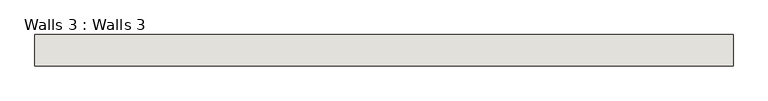
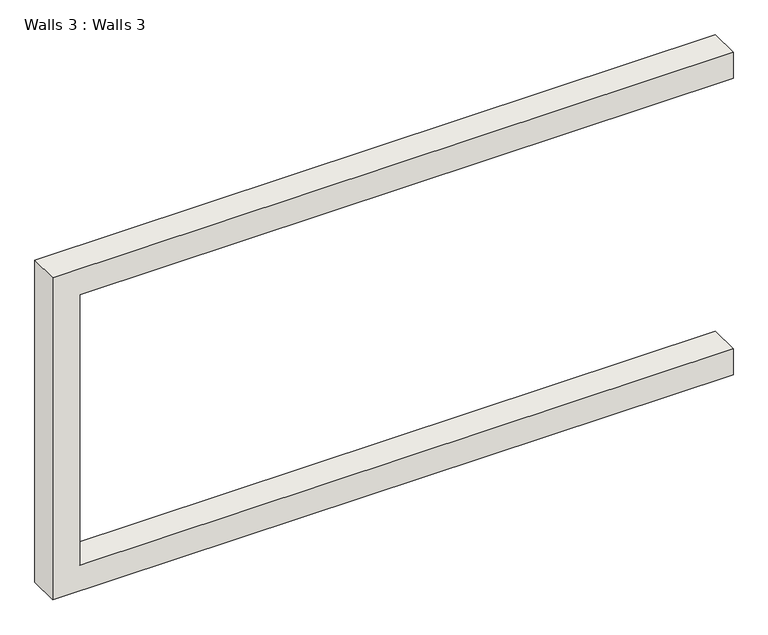
"""IFC4 building model written with IfcOpenShell, lengths in millimetres: wall geometry, Walls 3 : Walls 3."""

from ifc_helpers import new_model, si_unit, frame, origin, place, context, project, spatial, polyline, outline, extrude, source, transform, mapped, element, save


def walls_3_walls_3_aaa7465c(model_context):
    return source(origin(), model_context, "Body", "SweptSolid", [
        extrude(outline(polyline([(7623.0321664, -3925.6745124), (7623.0321664, -11850.4745124), (3657.6, -11850.4745124), (3657.6, -3925.6745124), (3973.3839769, -3925.6745124), (3973.3839769, -11535.2764802), (7302.5, -11535.2764802), (7302.5, -3925.6745124), (7623.0321664, -3925.6745124)])), frame((0.0, -900.5537077, 0.0), z_axis=(0.0, 1.0, 0.0), x_axis=(0.0, 0.0, 1.0)), (0.0, 0.0, 1.0), 354.8191178),
    ])


if __name__ == "__main__":
    model = new_model("IFC4")
    model_context = context("Model", 3, world=origin())
    ifc_project = project(units=[si_unit("LENGTHUNIT", "METRE", prefix="MILLI")], contexts=[model_context])
    site = spatial("IfcSite", under=ifc_project)
    building = spatial("IfcBuilding", under=site)
    placement = place(None, origin())
    walls_3_walls_3_shape = walls_3_walls_3_aaa7465c(model_context)
    element("IfcWall", 1, ObjectType="Walls 3 : Walls 3", at=placement, inside=building, context=model_context, shape_type="MappedRepresentation", body=[
        mapped(walls_3_walls_3_shape, transform((0.0, 0.0, 0.0), x_axis=(1.0, 0.0, 0.0), y_axis=(0.0, 1.0, 0.0), z_axis=(0.0, 0.0, 1.0))),
    ])
    save(model, "model.ifc")

# Revit data of these elements
# Element 1 (IfcWall, "Walls 3 : Walls 3")
#   Materials on its faces: "Default Wall"
# Materials
#   "Default Wall": colour RGB 128 128 128, transparency 0
